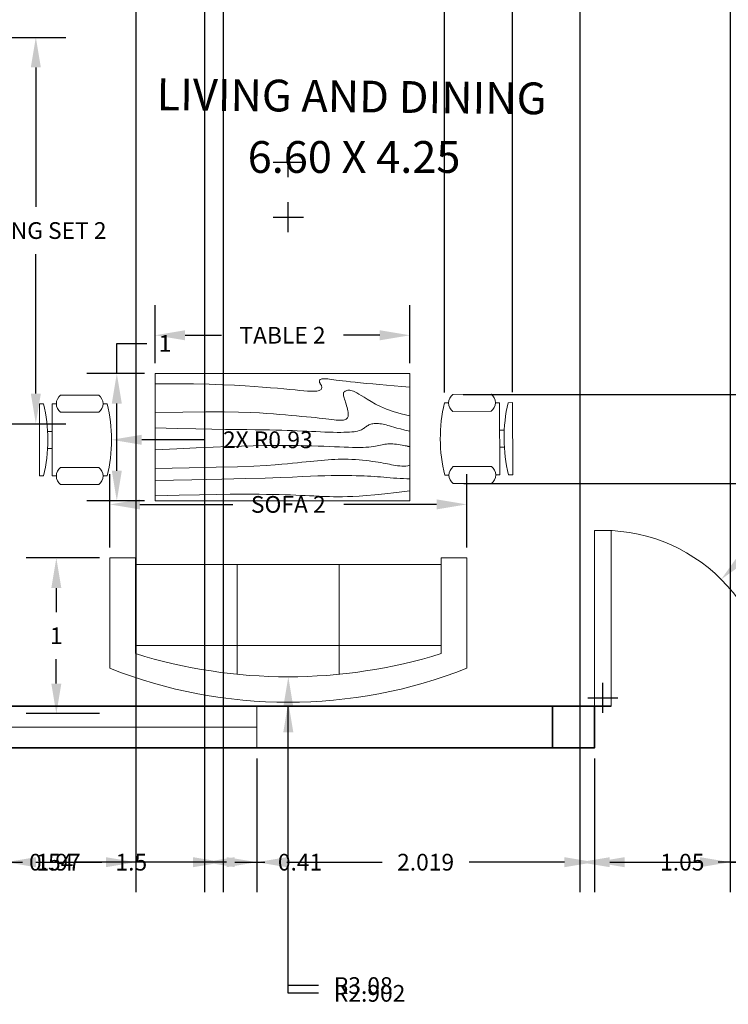
# Model space of a CAD drawing. Units: metres. Extents: x 180.3 to 196.1, y 135.7 to 166.1.
# Tile 2 of 5: x 183.3 to 187.5, y 150.2 to 156.1. Entities that reach past the tile are written whole.
import ezdxf

# ---------------------------------------------------------------- set-up
doc = ezdxf.new("R2010")
doc.units = ezdxf.units.M
doc.header["$MEASUREMENT"] = 0
for name, color, linetype, lineweight in [('A-ANNO-DIMS', 2, 'Continuous', 18), ('A-AREA-IDEN', 210, 'Continuous', 18), ('A-FURN', 190, 'Continuous', 18), ('A-GLAZ', 130, 'Continuous', 18), ('dim', 70, 'Continuous', 15), ('door', 240, 'Continuous', 18), ('wall', 50, 'Continuous', 35)]:
    doc.layers.add(name, color=color, linetype=linetype, lineweight=lineweight)
doc.styles.get("Standard").update_dxf_attribs({"font": 'arial.ttf', "height": 0.1})
doc.dimstyles.get("Standard").update_dxf_attribs({"dimtxt": 0.18, "dimasz": 0.18, "dimexe": 0.18, "dimexo": 0.0625, "dimgap": 0.09, "dimtad": 0, "dimtih": 1, "dimtoh": 1, "dimdec": 4, "dimzin": 0, "dimdsep": 46, "dimtxsty": 'Standard', "dimcen": 0.09, "dimadec": 0, "dimazin": 0, "dimtfac": 1, "dimtdec": 4, "dimtofl": 0, "dimtmove": 0, "dimatfit": 3, "dimfxl": 1, "dimtolj": 1, "dimtzin": 0, "dimarcsym": 0})

# ---------------------------------------------------------------- blocks, each defined once
blk = doc.blocks.new('Sofa - Roundback 7 ft.')
for p, q in [((-12.00002, -32.4421), (-12.00003, -6.5971)), ((11.99997, -32.4421), (11.99998, -6.5971)), ((-36.000027, -34), (-36.000027, -11.4696)), ((35.99998, -34), (35.99998, -11.4696)), ((-35.999844, -13.3819), (35.9998, -13.3819)), ((-36.000027, -32.4421), (35.99998, -32.4421))]:
    blk.add_line(p, q)
for points in [[(-36.000027, -34), (-42.000027, -34), (-42.000027, -8)], [(41.99998, -8), (41.99998, -34), (35.99998, -34)]]:
    blk.add_lwpolyline(points)
for centre, radius, start, end in [((0, -114.25), 114.25, 68.43141, 111.5686), ((-0.00001, -127.1968), 121.1968, 72.72033, 107.2797)]:
    blk.add_arc(centre, radius, start, end)
blk = doc.blocks.new('Table - Rectangular Woodgrain 60 x 30 in.')
for p, q in [((0, 0), (0, -30)), ((60, 0), (0, 0)), ((60, -30), (60, 0)), ((0, -30), (60, -30))]:
    blk.add_line(p, q)
for points in [[(0, -2.4), (4.8155, -2.418), (9.0302, -2.4688), (12.709, -2.5477), (15.9167, -2.65), (18.7181, -2.7711), (21.1781, -2.9063), (23.3616, -3.0508), (25.3333, -3.2), (27.1477, -3.3495), (28.8172, -3.4958), (30.3437, -3.636), (31.7291, -3.7667), (32.9756, -3.8849), (34.0849, -3.9875), (35.059, -4.0714), (35.9, -4.1334), (36.6114, -4.1711), (37.2041, -4.1854), (37.6906, -4.1779), (38.0833, -4.15), (38.3948, -4.1034), (38.6375, -4.0396), (38.8239, -3.9602), (38.9666, -3.8667), (39.0764, -3.7608), (39.1573, -3.6448), (39.2116, -3.521), (39.2416, -3.3917), (39.2498, -3.2593), (39.2385, -3.1261), (39.21, -2.9944), (39.1666, -2.8667), (39.111, -2.7447), (39.0468, -2.6281), (38.978, -2.5163), (38.9083, -2.4083), (38.8418, -2.3035), (38.7823, -2.201), (38.7337, -2.1001), (38.7, -2), (38.6844, -1.9003), (38.6875, -1.8021), (38.7094, -1.707), (38.75, -1.6167), (38.8094, -1.5326), (38.8875, -1.4563), (38.9844, -1.3893), (39.1, -1.3333), (39.2351, -1.2896), (39.3937, -1.2583), (39.5804, -1.2396), (39.8, -1.2333), (40.057, -1.2396), (40.3562, -1.2583), (40.7023, -1.2896), (41.1, -1.3333), (41.5547, -1.3895), (42.0755, -1.4573), (42.6721, -1.5361), (43.3542, -1.625), (44.1316, -1.7233), (45.014, -1.8302), (46.0114, -1.9449), (47.1333, -2.0667), (48.3862, -2.1947), (49.7625, -2.3281), (51.2513, -2.4663), (52.8416, -2.6083), (54.5226, -2.7535), (56.2833, -2.9011), (58.1127, -3.0501), (60, -3.2)], [(0, -9.2), (6.5759, -9.0858), (11.9385, -9.0365), (16.2527, -9.0418), (19.6833, -9.0917), (22.3952, -9.1759), (24.5531, -9.2844), (26.322, -9.4069), (27.8666, -9.5333), (29.3241, -9.6553), (30.7203, -9.7719), (32.0532, -9.8837), (33.3208, -9.9917), (34.5213, -10.0965), (35.6526, -10.199), (36.7128, -10.2999), (37.7, -10.4), (38.6129, -10.4996), (39.4531, -10.5969), (40.223, -10.6895), (40.925, -10.775), (41.5613, -10.8512), (42.1344, -10.9156), (42.6465, -10.966), (43.1, -11), (43.4976, -11.0158), (43.8437, -11.0136), (44.143, -10.9942), (44.4, -10.9583), (44.6195, -10.9069), (44.8062, -10.8406), (44.9648, -10.7603), (45.1, -10.6667), (45.2155, -10.5598), (45.3114, -10.4365), (45.3871, -10.2929), (45.4416, -10.125), (45.4743, -9.929), (45.4844, -9.7011), (45.4709, -9.4371), (45.4333, -9.1333), (45.3716, -8.7883), (45.2896, -8.4104), (45.1919, -8.0107), (45.0833, -7.6), (44.9685, -7.1893), (44.8521, -6.7896), (44.7388, -6.4117), (44.6333, -6.0667), (44.54, -5.7628), (44.4614, -5.4979), (44.4001, -5.2675), (44.3583, -5.0667), (44.3384, -4.8909), (44.3427, -4.7354), (44.3736, -4.5956), (44.4333, -4.4667), (44.5236, -4.3453), (44.6427, -4.2333), (44.7884, -4.1339), (44.9583, -4.05), (45.1501, -3.9849), (45.3614, -3.9417), (45.59, -3.9234), (45.8333, -3.9333), (46.0915, -3.9749), (46.3734, -4.0531), (46.6906, -4.1736), (47.0542, -4.3417), (47.4756, -4.5629), (47.9661, -4.8427), (48.5372, -5.1866), (49.2, -5.6), (49.9676, -6.0844), (50.8594, -6.625), (51.8965, -7.2031), (53.1, -7.8), (54.491, -8.3969), (56.0906, -8.975), (57.9199, -9.5156), (60, -10)], [(0, -12.8), (5.1847, -12.9322), (9.6213, -13.0323), (13.3963, -13.1059), (16.5958, -13.1583), (19.3063, -13.1952), (21.614, -13.2219), (23.6054, -13.2439), (25.3666, -13.2667), (26.9728, -13.2947), (28.4531, -13.3281), (29.8256, -13.3663), (31.1083, -13.4083), (32.3191, -13.4535), (33.476, -13.501), (34.597, -13.5501), (35.7, -13.6), (36.7984, -13.6497), (37.8875, -13.6979), (38.9578, -13.743), (40, -13.7833), (41.0047, -13.8174), (41.9625, -13.8438), (42.864, -13.8607), (43.7, -13.8667), (44.4631, -13.8604), (45.1552, -13.8417), (45.7801, -13.8104), (46.3416, -13.7667), (46.8439, -13.7104), (47.2906, -13.6417), (47.6858, -13.5604), (48.0333, -13.4667), (48.3375, -13.3608), (48.6042, -13.2448), (48.8396, -13.121), (49.05, -12.9917), (49.2417, -12.8593), (49.4208, -12.7261), (49.5937, -12.5944), (49.7667, -12.4667), (49.9452, -12.3451), (50.1323, -12.2313), (50.3303, -12.1268), (50.5416, -12.0333), (50.7686, -11.9524), (51.0135, -11.8854), (51.2788, -11.8341), (51.5666, -11.8), (51.8785, -11.7843), (52.2116, -11.7865), (52.562, -11.8059), (52.926, -11.8417), (53.2998, -11.8931), (53.6795, -11.9594), (54.0614, -12.0397), (54.4416, -12.1333), (54.8223, -12.2401), (55.2293, -12.3625), (55.6942, -12.5037), (56.2489, -12.6667), (56.9251, -12.8547), (57.7545, -13.0708), (58.7689, -13.3182), (60, -13.6)], [(0, -18), (5.124, -17.7273), (9.6609, -17.5057), (13.6705, -17.3303), (17.2125, -17.1958), (20.3467, -17.0973), (23.1328, -17.0297), (25.6307, -16.9878), (27.9, -16.9667), (29.9928, -16.9617), (31.9302, -16.9703), (33.7254, -16.9907), (35.3917, -17.0208), (36.9423, -17.0588), (38.3906, -17.1026), (39.7499, -17.1503), (41.0333, -17.2), (42.2519, -17.2496), (43.4073, -17.2969), (44.4986, -17.3395), (45.525, -17.375), (46.4858, -17.4012), (47.3802, -17.4156), (48.2074, -17.416), (48.9667, -17.4), (49.6583, -17.3662), (50.2872, -17.3167), (50.8595, -17.2547), (51.3812, -17.1833), (51.8584, -17.1057), (52.2971, -17.025), (52.7034, -16.9443), (53.0833, -16.8667), (53.443, -16.7951), (53.789, -16.7313), (54.128, -16.6768), (54.4666, -16.6334), (54.8115, -16.6024), (55.1693, -16.5854), (55.5465, -16.5841), (55.95, -16.6), (56.3828, -16.6337), (56.8346, -16.6823), (57.2915, -16.7418), (57.7396, -16.8084), (58.165, -16.878), (58.5539, -16.9469), (58.8924, -17.0111), (59.1666, -17.0667), (59.3679, -17.1107), (59.5078, -17.1438), (59.6032, -17.1675), (59.6708, -17.1833), (59.7275, -17.193), (59.7901, -17.1979), (59.8753, -17.1998), (60, -17.2)], [(0, -22.4), (8.0098, -22.2501), (14.4094, -22.1011), (19.4168, -21.9535), (23.25, -21.8083), (26.1269, -21.6663), (28.2656, -21.5281), (29.884, -21.3947), (31.2, -21.2667), (32.3967, -21.1448), (33.5172, -21.0292), (34.5697, -20.9198), (35.5625, -20.8167), (36.5037, -20.7198), (37.4015, -20.6292), (38.2642, -20.5448), (39.1, -20.4667), (39.9164, -20.3951), (40.7187, -20.3313), (41.5117, -20.2768), (42.3, -20.2333), (43.0883, -20.2024), (43.8812, -20.1854), (44.6836, -20.1841), (45.5, -20.2), (46.3328, -20.234), (47.1747, -20.2844), (48.0163, -20.3488), (48.8479, -20.425), (49.66, -20.5106), (50.4429, -20.6031), (51.1872, -20.7004), (51.8833, -20.8), (52.5246, -20.8999), (53.1166, -20.9995), (53.6681, -21.0983), (54.1875, -21.1958), (54.6834, -21.2919), (55.1646, -21.3859), (55.6394, -21.4777), (56.1167, -21.5667), (56.6028, -21.6515), (57.0961, -21.7266), (57.5929, -21.7852), (58.0896, -21.8208), (58.5823, -21.8268), (59.0674, -21.7964), (59.5412, -21.723), (60, -21.6)], [(0, -25.2), (8.6355, -25.0504), (15.7026, -24.9031), (21.4049, -24.7606), (25.9458, -24.625), (29.529, -24.4988), (32.3578, -24.3844), (34.6359, -24.284), (36.5667, -24.2), (38.3213, -24.1341), (39.9417, -24.0854), (41.437, -24.0523), (42.8167, -24.0333), (44.0901, -24.0268), (45.2667, -24.0313), (46.3557, -24.0451), (47.3667, -24.0667), (48.309, -24.0947), (49.1928, -24.1287), (50.0284, -24.168), (50.826, -24.2125), (51.5959, -24.2617), (52.3483, -24.3151), (53.0935, -24.3725), (53.8417, -24.4334), (54.6009, -24.497), (55.3699, -24.561), (56.1454, -24.6226), (56.9239, -24.6792), (57.7021, -24.7279), (58.4764, -24.7662), (59.2435, -24.7911), (60, -24.8)], [(0, -28.8), (5.6867, -28.6681), (10.45, -28.5698), (14.407, -28.5012), (17.675, -28.4584), (20.3711, -28.4374), (22.6125, -28.4344), (24.5164, -28.4455), (26.2, -28.4667), (27.762, -28.4947), (29.2276, -28.5281), (30.6033, -28.5663), (31.8958, -28.6084), (33.1118, -28.6535), (34.2578, -28.7011), (35.3405, -28.7501), (36.3666, -28.8), (37.3443, -28.8497), (38.288, -28.8974), (39.2137, -28.9412), (40.1375, -28.9792), (41.0753, -29.0093), (42.0432, -29.0297), (43.0572, -29.0384), (44.1333, -29.0333), (45.2936, -29.0114), (46.5843, -28.9641), (48.0579, -28.8816), (49.7666, -28.7542), (51.7629, -28.5721), (54.0989, -28.3255), (56.8272, -28.0048), (60, -27.6)]]:
    blk.add_lwpolyline(points)
blk = doc.blocks.new('Chair - Desk')
for p, q in [((-8.5, 0), (-8.5, -1)), ((-8.5, 0), (8.5, 0)), ((8.5, 0), (8.5, -1)), ((-2, -3), (-2, -1.9355)), ((2, -1.9576), (2, -3)), ((-8.5, -3), (-8.5, -4)), ((-8.5, -3), (8.5, -3)), ((8.5, -3), (8.5, -4)), ((-10.5, -5), (-10.5, -14)), ((-6.5, -14), (-6.5, -5)), ((6.5, -5), (6.5, -14)), ((10.5, -14), (10.5, -5)), ((-8.5, -15), (-8.5, -16)), ((8.5, -15), (8.5, -16))]:
    blk.add_line(p, q)
for centre, radius, start, end in [((0, 34.625), 36.625, 256.5803, 283.4197), ((-8.5, -6.5), 2.5, 36.8699, 143.1301), ((8.5, -6.5), 2.5, 36.8699, 143.1301), ((-8.5, -12.5), 2.5, 216.8699, 323.1301), ((0, 19.625), 36.625, 256.5803, 283.4197), ((8.5, -12.5), 2.5, 216.8699, 323.1301)]:
    blk.add_arc(centre, radius, start, end)
blk = doc.blocks.new('DOOR-1050')
for p, q in [((0.0004, -0.0001), (0.0004, 1.0499)), ((0.1004, -0.0001), (0.1004, 1.0499))]:
    blk.add_line(p, q)
blk.add_arc((0.0504, 0.0499), 1.0012, 357.13759, 92.86241)
blk = doc.blocks.new('WIN-1500')
for p, q in [((0.0003, 0.2499), (0.0003, -0.0001)), ((1.5003, 0.2499), (1.5003, -0.0001)), ((1.5003, 0.1249), (0.0003, 0.1249))]:
    blk.add_line(p, q)
blk = doc.blocks.new('*D25')
at = {"layer": 'A-ANNO-DIMS', "color": 0, "lineweight": -2, "transparency": 16777216}
for p, q in [((183.1113, 155.9984), (183.5755, 155.9984)), ((183.3955, 155.8184), (183.3955, 154.9844)), ((183.3955, 153.867), (183.3955, 154.701)), ((183.1113, 153.687), (183.5755, 153.687))]:
    blk.add_line(p, q, dxfattribs=at)
at = {"layer": 'A-ANNO-DIMS', "color": 0, "transparency": 16777216}
for points in [[(183.3655, 155.8184), (183.4255, 155.8184), (183.3955, 155.9984)], [(183.3655, 153.867), (183.4255, 153.867), (183.3955, 153.687)]]:
    blk.add_solid(points, dxfattribs=at)
at = {"layer": 'Defpoints', "color": 0, "transparency": 16777216}
for p in [(183.0488, 155.9984), (183.0488, 153.687), (183.3955, 153.687)]:
    blk.add_point(p, dxfattribs=at)
at = {"layer": 'A-ANNO-DIMS', "color": 0, "transparency": 16777216, "insert": (183.3955, 154.8427), "char_height": 0.1, "attachment_point": 5}
blk.add_mtext('\\A1;DINING SET 2', dxfattribs=at)
blk = doc.blocks.new('*D27')
at = {"layer": 'A-ANNO-DIMS', "color": 0, "lineweight": -2, "transparency": 16777216}
for p, q in [((183.8381, 152.9469), (183.8381, 153.3845)), ((185.9717, 152.9469), (185.9717, 153.3845)), ((184.0181, 153.2045), (184.5733, 153.2045)), ((185.7917, 153.2045), (185.2365, 153.2045))]:
    blk.add_line(p, q, dxfattribs=at)
at = {"layer": 'A-ANNO-DIMS', "color": 0, "transparency": 16777216}
for points in [[(184.0181, 153.2345), (184.0181, 153.1745), (183.8381, 153.2045)], [(185.7917, 153.2345), (185.7917, 153.1745), (185.9717, 153.2045)]]:
    blk.add_solid(points, dxfattribs=at)
at = {"layer": 'Defpoints', "color": 0, "transparency": 16777216}
for p in [(183.8381, 153.2045), (183.8381, 152.8844), (185.9717, 152.8844)]:
    blk.add_point(p, dxfattribs=at)
at = {"layer": 'A-ANNO-DIMS', "color": 0, "transparency": 16777216, "insert": (184.9049, 153.2045), "char_height": 0.1, "attachment_point": 5}
blk.add_mtext('\\A1;SOFA 2', dxfattribs=at)
blk = doc.blocks.new('*D28')
at = {"layer": 'A-ANNO-DIMS', "color": 0, "lineweight": -2, "transparency": 16777216}
for p, q in [((183.7756, 152.8844), (183.3381, 152.8844)), ((183.5181, 152.7044), (183.5181, 152.559)), ((183.5181, 152.1331), (183.5181, 152.2786)), ((183.7756, 151.9531), (183.3381, 151.9531))]:
    blk.add_line(p, q, dxfattribs=at)
at = {"layer": 'A-ANNO-DIMS', "color": 0, "transparency": 16777216}
for points in [[(183.4881, 152.7044), (183.5481, 152.7044), (183.5181, 152.8844)], [(183.4881, 152.1331), (183.5481, 152.1331), (183.5181, 151.9531)]]:
    blk.add_solid(points, dxfattribs=at)
at = {"layer": 'Defpoints', "color": 0, "transparency": 16777216}
for p in [(183.8381, 152.8844), (183.5181, 151.9531), (183.8381, 151.9531)]:
    blk.add_point(p, dxfattribs=at)
at = {"layer": 'A-ANNO-DIMS', "color": 0, "transparency": 16777216, "insert": (183.5181, 152.4188), "char_height": 0.1, "attachment_point": 5}
blk.add_mtext('\\A1;1', dxfattribs=at)
blk = doc.blocks.new('*D29')
at = {"layer": 'A-ANNO-DIMS', "color": 0, "lineweight": -2, "transparency": 16777216}
for p, q in [((184.1082, 154.0502), (184.1082, 154.3963)), ((185.6322, 154.0502), (185.6322, 154.3963)), ((184.2882, 154.2163), (184.506, 154.2163)), ((185.4522, 154.2163), (185.2345, 154.2163))]:
    blk.add_line(p, q, dxfattribs=at)
at = {"layer": 'A-ANNO-DIMS', "color": 0, "transparency": 16777216}
for points in [[(184.2882, 154.2463), (184.2882, 154.1863), (184.1082, 154.2163)], [(185.4522, 154.2463), (185.4522, 154.1863), (185.6322, 154.2163)]]:
    blk.add_solid(points, dxfattribs=at)
at = {"layer": 'Defpoints', "color": 0, "transparency": 16777216}
for p in [(185.6322, 154.2163), (184.1082, 153.9877), (185.6322, 153.9877)]:
    blk.add_point(p, dxfattribs=at)
at = {"layer": 'A-ANNO-DIMS', "color": 0, "transparency": 16777216, "insert": (184.8702, 154.2163), "char_height": 0.1, "attachment_point": 5}
blk.add_mtext('\\A1;TABLE 2', dxfattribs=at)
blk = doc.blocks.new('*D30')
at = {"layer": 'A-ANNO-DIMS', "color": 0, "lineweight": -2, "transparency": 16777216}
for p, q in [((183.8796, 153.9877), (183.8796, 154.1677)), ((183.8796, 154.1677), (184.0596, 154.1677)), ((184.0457, 153.9877), (183.6996, 153.9877)), ((183.8796, 153.4057), (183.8796, 153.8077)), ((184.0457, 153.2257), (183.6996, 153.2257))]:
    blk.add_line(p, q, dxfattribs=at)
at = {"layer": 'A-ANNO-DIMS', "color": 0, "transparency": 16777216}
for points in [[(183.8496, 153.8077), (183.9096, 153.8077), (183.8796, 153.9877)], [(183.8496, 153.4057), (183.9096, 153.4057), (183.8796, 153.2257)]]:
    blk.add_solid(points, dxfattribs=at)
at = {"layer": 'Defpoints', "color": 0, "transparency": 16777216}
for p in [(183.8796, 153.9877), (184.1082, 153.9877), (184.1082, 153.2257)]:
    blk.add_point(p, dxfattribs=at)
at = {"layer": 'A-ANNO-DIMS', "color": 0, "transparency": 16777216, "insert": (184.1681, 154.1677), "char_height": 0.1, "attachment_point": 5}
blk.add_mtext('\\A1;1', dxfattribs=at)
blk = doc.blocks.new('*D40')
at = {"layer": 'A-ANNO-DIMS', "color": 0, "lineweight": -2, "transparency": 16777216}
for p, q in [((183.2164, 151.6854), (183.2164, 150.8842)), ((184.7164, 151.6854), (184.7164, 150.8842)), ((183.3964, 151.0642), (183.7897, 151.0642)), ((184.5364, 151.0642), (184.1431, 151.0642))]:
    blk.add_line(p, q, dxfattribs=at)
at = {"layer": 'A-ANNO-DIMS', "color": 0, "transparency": 16777216}
for points in [[(183.3964, 151.0942), (183.3964, 151.0342), (183.2164, 151.0642)], [(184.5364, 151.0942), (184.5364, 151.0342), (184.7164, 151.0642)]]:
    blk.add_solid(points, dxfattribs=at)
at = {"layer": 'Defpoints', "color": 0, "transparency": 16777216}
for p in [(183.2164, 151.7479), (184.7164, 151.7479), (184.7164, 151.0642)]:
    blk.add_point(p, dxfattribs=at)
at = {"layer": 'A-ANNO-DIMS', "color": 0, "transparency": 16777216, "insert": (183.9664, 151.0642), "char_height": 0.1, "attachment_point": 5}
blk.add_mtext('\\A1;1.5', dxfattribs=at)
blk = doc.blocks.new('*D41')
at = {"layer": 'A-ANNO-DIMS', "color": 0, "lineweight": -2, "transparency": 16777216}
for p, q in [((184.7164, 151.6854), (184.7164, 150.8842)), ((186.7354, 151.6854), (186.7354, 150.8842)), ((184.8964, 151.0642), (185.4662, 151.0642)), ((186.5554, 151.0642), (185.9856, 151.0642))]:
    blk.add_line(p, q, dxfattribs=at)
at = {"layer": 'A-ANNO-DIMS', "color": 0, "transparency": 16777216}
for points in [[(184.8964, 151.0942), (184.8964, 151.0342), (184.7164, 151.0642)], [(186.5554, 151.0942), (186.5554, 151.0342), (186.7354, 151.0642)]]:
    blk.add_solid(points, dxfattribs=at)
at = {"layer": 'Defpoints', "color": 0, "transparency": 16777216}
for p in [(184.7164, 151.7479), (186.7354, 151.7479), (186.7354, 151.0642)]:
    blk.add_point(p, dxfattribs=at)
at = {"layer": 'A-ANNO-DIMS', "color": 0, "transparency": 16777216, "insert": (185.7259, 151.0642), "char_height": 0.1, "attachment_point": 5}
blk.add_mtext('\\A1;2.019', dxfattribs=at)
blk = doc.blocks.new('*D42')
at = {"layer": 'A-ANNO-DIMS', "color": 0, "lineweight": -2, "transparency": 16777216}
for p, q in [((186.7354, 151.6854), (186.7354, 150.8842)), ((187.7854, 151.6854), (187.7854, 150.8842)), ((186.9154, 151.0642), (187.0449, 151.0642)), ((187.6054, 151.0642), (187.476, 151.0642))]:
    blk.add_line(p, q, dxfattribs=at)
at = {"layer": 'A-ANNO-DIMS', "color": 0, "transparency": 16777216}
for points in [[(186.9154, 151.0942), (186.9154, 151.0342), (186.7354, 151.0642)], [(187.6054, 151.0942), (187.6054, 151.0342), (187.7854, 151.0642)]]:
    blk.add_solid(points, dxfattribs=at)
at = {"layer": 'Defpoints', "color": 0, "transparency": 16777216}
for p in [(186.7354, 151.7479), (187.7854, 151.7479), (187.7854, 151.0642)]:
    blk.add_point(p, dxfattribs=at)
at = {"layer": 'A-ANNO-DIMS', "color": 0, "transparency": 16777216, "insert": (187.2604, 151.0642), "char_height": 0.1, "attachment_point": 5}
blk.add_mtext('\\A1;1.05', dxfattribs=at)
blk = doc.blocks.new('*D51')
at = {"layer": 'A-ANNO-DIMS', "color": 0, "lineweight": -2, "transparency": 16777216}
for p, q in [((182.5473, 156.4354), (182.5473, 150.8842)), ((183.0878, 156.4354), (183.0878, 150.8842)), ((182.7273, 151.0642), (182.9078, 151.0642)), ((183.0878, 151.0642), (183.2678, 151.0642))]:
    blk.add_line(p, q, dxfattribs=at)
at = {"layer": 'A-ANNO-DIMS', "color": 0, "transparency": 16777216}
for points in [[(182.7273, 151.0942), (182.7273, 151.0342), (182.5473, 151.0642)], [(182.9078, 151.0942), (182.9078, 151.0342), (183.0878, 151.0642)]]:
    blk.add_solid(points, dxfattribs=at)
at = {"layer": 'Defpoints', "color": 0, "transparency": 16777216}
for p in [(182.5473, 156.4979), (183.0878, 156.4979), (183.0878, 151.0642)]:
    blk.add_point(p, dxfattribs=at)
at = {"layer": 'A-ANNO-DIMS', "color": 0, "transparency": 16777216, "insert": (183.4875, 151.0642), "char_height": 0.1, "attachment_point": 5}
blk.add_mtext('\\A1;0.54', dxfattribs=at)
blk = doc.blocks.new('*D52')
at = {"layer": 'A-ANNO-DIMS', "color": 0, "lineweight": -2, "transparency": 16777216}
for p, q in [((182.5473, 158.3772), (182.5473, 150.8842)), ((184.5151, 158.3772), (184.5151, 150.8842)), ((182.7273, 151.0642), (183.316, 151.0642)), ((184.3351, 151.0642), (183.7464, 151.0642))]:
    blk.add_line(p, q, dxfattribs=at)
at = {"layer": 'A-ANNO-DIMS', "color": 0, "transparency": 16777216}
for points in [[(182.7273, 151.0942), (182.7273, 151.0342), (182.5473, 151.0642)], [(184.3351, 151.0942), (184.3351, 151.0342), (184.5151, 151.0642)]]:
    blk.add_solid(points, dxfattribs=at)
at = {"layer": 'Defpoints', "color": 0, "transparency": 16777216}
for p in [(182.5473, 158.4397), (184.5151, 158.4397), (184.5151, 151.0642)]:
    blk.add_point(p, dxfattribs=at)
at = {"layer": 'A-ANNO-DIMS', "color": 0, "transparency": 16777216, "insert": (183.5312, 151.0642), "char_height": 0.1, "attachment_point": 5}
blk.add_mtext('\\A1;1.97', dxfattribs=at)
blk = doc.blocks.new('*D54')
at = {"layer": 'A-ANNO-DIMS', "color": 0, "lineweight": -2, "transparency": 16777216}
for p, q in [((186.6473, 162.1854), (186.6473, 150.8842)), ((187.5473, 162.1854), (187.5473, 150.8842)), ((186.8273, 151.0642), (187.3673, 151.0642)), ((187.5473, 151.0642), (187.7273, 151.0642))]:
    blk.add_line(p, q, dxfattribs=at)
at = {"layer": 'A-ANNO-DIMS', "color": 0, "transparency": 16777216}
for points in [[(186.8273, 151.0942), (186.8273, 151.0342), (186.6473, 151.0642)], [(187.3673, 151.0942), (187.3673, 151.0342), (187.5473, 151.0642)]]:
    blk.add_solid(points, dxfattribs=at)
at = {"layer": 'Defpoints', "color": 0, "transparency": 16777216}
for p in [(186.6473, 162.2479), (187.5473, 162.2479), (187.5473, 151.0642)]:
    blk.add_point(p, dxfattribs=at)
at = {"layer": 'A-ANNO-DIMS', "color": 0, "transparency": 16777216, "insert": (187.9085, 151.0642), "char_height": 0.1, "attachment_point": 5}
blk.add_mtext('\\A1;0.9', dxfattribs=at)
blk = doc.blocks.new('*D61')
at = {"layer": 'A-ANNO-DIMS', "color": 0, "lineweight": -2, "transparency": 16777216}
for p, q in [((183.9941, 158.6956), (183.9941, 150.8842)), ((184.4049, 158.6956), (184.4049, 150.8842)), ((183.8141, 151.0642), (183.6341, 151.0642)), ((184.5849, 151.0642), (184.7649, 151.0642))]:
    blk.add_line(p, q, dxfattribs=at)
at = {"layer": 'A-ANNO-DIMS', "color": 0, "transparency": 16777216}
for points in [[(183.8141, 151.0942), (183.8141, 151.0342), (183.9941, 151.0642)], [(184.5849, 151.0942), (184.5849, 151.0342), (184.4049, 151.0642)]]:
    blk.add_solid(points, dxfattribs=at)
at = {"layer": 'Defpoints', "color": 0, "transparency": 16777216}
for p in [(183.9941, 158.7581), (184.4049, 158.7581), (184.4049, 151.0642)]:
    blk.add_point(p, dxfattribs=at)
at = {"layer": 'A-ANNO-DIMS', "color": 0, "transparency": 16777216, "insert": (184.9751, 151.0642), "char_height": 0.1, "attachment_point": 5}
blk.add_mtext('\\A1;0.41', dxfattribs=at)
blk = doc.blocks.new('*D63')
at = {"layer": 'A-ANNO-DIMS', "color": 0, "lineweight": -2, "transparency": 16777216}
for p, q in [((185.8382, 153.8738), (185.8382, 166.1117)), ((186.2446, 153.8757), (186.2446, 166.1117)), ((185.6582, 165.9317), (185.4782, 165.9317)), ((186.4246, 165.9317), (186.6046, 165.9317))]:
    blk.add_line(p, q, dxfattribs=at)
at = {"layer": 'A-ANNO-DIMS', "color": 0, "transparency": 16777216}
for points in [[(185.6582, 165.9617), (185.6582, 165.9017), (185.8382, 165.9317)], [(186.4246, 165.9617), (186.4246, 165.9017), (186.2446, 165.9317)]]:
    blk.add_solid(points, dxfattribs=at)
at = {"layer": 'Defpoints', "color": 0, "transparency": 16777216}
for p in [(186.2446, 165.9317), (185.8382, 153.8113), (186.2446, 153.8132)]:
    blk.add_point(p, dxfattribs=at)
at = {"layer": 'A-ANNO-DIMS', "color": 0, "transparency": 16777216, "insert": (186.8148, 165.9317), "char_height": 0.1, "attachment_point": 5}
blk.add_mtext('\\A1;0.41', dxfattribs=at)
blk = doc.blocks.new('*D64')
at = {"layer": 'A-ANNO-DIMS', "color": 0, "lineweight": -2, "transparency": 16777216}
for p, q in [((195.531085, 154.042344), (195.531085, 154.222344)), ((185.951216, 153.862344), (195.711085, 153.862344)), ((185.953765, 153.32895), (195.711085, 153.32895)), ((195.531085, 153.14895), (195.531085, 152.96895))]:
    blk.add_line(p, q, dxfattribs=at)
at = {"layer": 'A-ANNO-DIMS', "color": 0, "transparency": 16777216}
for points in [[(195.501085, 154.042344), (195.561085, 154.042344), (195.531085, 153.862344)], [(195.501085, 153.14895), (195.561085, 153.14895), (195.531085, 153.32895)]]:
    blk.add_solid(points, dxfattribs=at)
at = {"layer": 'Defpoints', "color": 0, "transparency": 16777216}
for p in [(185.888716, 153.862344), (195.531085, 153.862344), (185.891265, 153.32895)]:
    blk.add_point(p, dxfattribs=at)
at = {"layer": 'A-ANNO-DIMS', "color": 0, "transparency": 16777216, "insert": (195.531085, 153.595647), "char_height": 0.1, "attachment_point": 5}
blk.add_mtext('\\A1;0.53', dxfattribs=at)
blk = doc.blocks.new('*D66')
at = {"layer": 'A-ANNO-DIMS', "color": 0, "lineweight": -2, "transparency": 16777216}
for p, q in [((187.9178, 153.1811), (187.6204, 152.8835)), ((188.0978, 153.1811), (187.9178, 153.1811)), ((186.7854, 151.9579), (186.7854, 152.1379)), ((186.6954, 152.0479), (186.8754, 152.0479))]:
    blk.add_line(p, q, dxfattribs=at)
at = {"layer": 'A-ANNO-DIMS', "color": 0, "transparency": 16777216}
blk.add_solid([(187.5992, 152.9047), (187.6416, 152.8623), (187.4932, 152.7562)], dxfattribs=at)
at = {"layer": 'Defpoints', "color": 0, "transparency": 16777216}
for p in [(187.4932, 152.7562), (186.7854, 152.0479)]:
    blk.add_point(p, dxfattribs=at)
at = {"layer": 'A-ANNO-DIMS', "color": 0, "transparency": 16777216, "insert": (188.4748, 153.1811), "char_height": 0.1, "attachment_point": 5}
blk.add_mtext('\\A1;4X R1.00', dxfattribs=at)
blk = doc.blocks.new('*D69')
at = {"layer": 'A-ANNO-DIMS', "color": 0, "lineweight": -2, "transparency": 16777216}
for p, q in [((182.9181, 153.5006), (182.9181, 153.6806)), ((182.8281, 153.5906), (183.0081, 153.5906)), ((184.4065, 153.5912), (184.0284, 153.5911))]:
    blk.add_line(p, q, dxfattribs=at)
at = {"layer": 'A-ANNO-DIMS', "color": 0, "transparency": 16777216}
blk.add_solid([(184.0284, 153.6211), (184.0284, 153.5611), (183.8484, 153.591)], dxfattribs=at)
at = {"layer": 'Defpoints', "color": 0, "transparency": 16777216}
for p in [(182.9181, 153.5906), (183.8484, 153.591)]:
    blk.add_point(p, dxfattribs=at)
at = {"layer": 'A-ANNO-DIMS', "color": 0, "transparency": 16777216, "insert": (184.7826, 153.5912), "char_height": 0.1, "attachment_point": 5}
blk.add_mtext('\\A1;2X R0.93', dxfattribs=at)
blk = doc.blocks.new('*D70')
at = {"layer": 'A-ANNO-DIMS', "color": 0, "lineweight": -2, "transparency": 16777216}
for p, q in [((184.9049, 155.1616), (184.9049, 155.3416)), ((184.8149, 155.2516), (184.9949, 155.2516)), ((184.905, 150.3262), (184.905, 151.9932)), ((185.085, 150.3262), (184.905, 150.3262))]:
    blk.add_line(p, q, dxfattribs=at)
at = {"layer": 'A-ANNO-DIMS', "color": 0, "transparency": 16777216}
blk.add_solid([(184.935, 151.9932), (184.875, 151.9932), (184.905, 152.1732)], dxfattribs=at)
at = {"layer": 'Defpoints', "color": 0, "transparency": 16777216}
for p in [(184.9049, 155.2516), (184.905, 152.1732)]:
    blk.add_point(p, dxfattribs=at)
at = {"layer": 'A-ANNO-DIMS', "color": 0, "transparency": 16777216, "insert": (185.3529, 150.3262), "char_height": 0.1, "attachment_point": 5}
blk.add_mtext('\\A1;R3.08', dxfattribs=at)
blk = doc.blocks.new('*D71')
at = {"layer": 'A-ANNO-DIMS', "color": 0, "lineweight": -2, "transparency": 16777216}
for p, q in [((184.9049, 154.8328), (184.9049, 155.0128)), ((184.8149, 154.9228), (184.9949, 154.9228)), ((184.905, 150.2797), (184.905, 151.8408)), ((185.085, 150.2797), (184.905, 150.2797))]:
    blk.add_line(p, q, dxfattribs=at)
at = {"layer": 'A-ANNO-DIMS', "color": 0, "transparency": 16777216}
blk.add_solid([(184.935, 151.8408), (184.875, 151.8408), (184.905, 152.0208)], dxfattribs=at)
at = {"layer": 'Defpoints', "color": 0, "transparency": 16777216}
for p in [(184.9049, 154.9228), (184.905, 152.0208)]:
    blk.add_point(p, dxfattribs=at)
at = {"layer": 'A-ANNO-DIMS', "color": 0, "transparency": 16777216, "insert": (185.3911, 150.2797), "char_height": 0.1, "attachment_point": 5}
blk.add_mtext('\\A1;R2.902', dxfattribs=at)

msp = doc.modelspace()

# ---------------------------------------------------------------- linework, layer by layer
at = {"layer": 'wall'}
for p, q in [((186.8354, 151.9979), (181.4473, 151.9979)), ((186.7354, 151.7479), (181.1973, 151.7479))]:
    msp.add_line(p, q, dxfattribs=at)
msp.add_lwpolyline([(186.4854, 151.9979), (186.7354, 151.9979), (186.7354, 151.7479), (186.4854, 151.7479)], close=True, dxfattribs=at)

# ---------------------------------------------------------------- block references
at = {"layer": 'A-FURN', "xscale": 0.0254, "yscale": 0.0254, "zscale": 0.0254}
msp.add_blockref('Table - Rectangular Woodgrain 60 x 30 in.', (184.1082, 153.9877), dxfattribs=at)
at = {"layer": 'A-FURN', "yscale": 0.0254, "zscale": 0.0254}
for name, p, xscale, rotation in [('Chair - Desk', (183.4166, 153.5906), 0.0254, 90), ('Chair - Desk', (186.2456, 153.5973), -0.0254, 270.2737751839787), ('Sofa - Roundback 7 ft.', (184.9049, 152.0208), 0.0254, 180)]:
    msp.add_blockref(name, p, dxfattribs=dict(at, xscale=xscale, rotation=rotation))
at = {"layer": 'A-GLAZ'}
msp.add_blockref('WIN-1500', (183.216, 151.748), dxfattribs=at)
at = {"layer": 'door'}
msp.add_blockref('DOOR-1050', (186.735, 151.998), dxfattribs=at)

# ---------------------------------------------------------------- texts
at = {"layer": 'A-AREA-IDEN', "insert": (183.198, 155.7632), "char_height": 0.19, "attachment_point": 1, "rotation": 359.37384}
msp.add_mtext_dynamic_manual_height_columns('\\pxqc;LIVING AND DINING ', width=4.172977, gutter_width=1, heights=[0], dxfattribs=at)
at = {"layer": 'dim', "insert": (183.8767, 155.3779), "char_height": 0.19, "attachment_point": 1}
msp.add_mtext_dynamic_manual_height_columns('\\pxqc;6.60 X 4.25', width=2.842675, gutter_width=1, heights=[0], dxfattribs=at)

# ---------------------------------------------------------------- dimensions: what is measured, and where the dimension line sits
at = {"layer": 'A-ANNO-DIMS'}
for base, p1, p2, override, picture, middle in [((186.2446, 165.9317), (185.8382, 153.8113), (186.2446, 153.8132), {"dimdec": 2, "dimlfac": 1, "dimrnd": 0, "dimzin": 0, "dimdsep": 46, "dimlunit": 2}, '*D63', (186.8148, 165.9317)), ((187.5473, 151.0642), (186.6473, 162.2479), (187.5473, 162.2479), {"dimdec": 1, "dimlfac": 1, "dimrnd": 0, "dimzin": 0, "dimdsep": 46, "dimlunit": 2}, '*D54', (187.9085, 151.0642)), ((184.4049, 151.0642), (183.9941, 158.7581), (184.4049, 158.7581), {"dimdec": 2, "dimlfac": 1, "dimrnd": 0, "dimzin": 0, "dimdsep": 46, "dimlunit": 2}, '*D61', (184.9751, 151.0642)), ((184.5151, 151.0642), (182.5473, 158.4397), (184.5151, 158.4397), {"dimdec": 2, "dimlfac": 1, "dimrnd": 0, "dimzin": 0, "dimdsep": 46, "dimlunit": 2}, '*D52', (183.5312, 151.0642)), ((183.0878, 151.0642), (182.5473, 156.4979), (183.0878, 156.4979), {"dimdec": 2, "dimlfac": 1, "dimrnd": 0, "dimzin": 0, "dimdsep": 46, "dimlunit": 2}, '*D51', (183.4875, 151.0642)), ((184.7164, 151.0642), (183.2164, 151.7479), (184.7164, 151.7479), {"dimdec": 1, "dimlfac": 1, "dimrnd": 0, "dimzin": 0, "dimdsep": 46, "dimlunit": 2}, '*D40', (183.9664, 151.0642)), ((186.7354, 151.0642), (184.7164, 151.7479), (186.7354, 151.7479), {"dimdec": 3, "dimlfac": 1, "dimrnd": 0, "dimzin": 0, "dimdsep": 46, "dimlunit": 2}, '*D41', (185.7259, 151.0642)), ((187.7854, 151.0642), (186.7354, 151.7479), (187.7854, 151.7479), {"dimdec": 2, "dimlfac": 1, "dimrnd": 0, "dimzin": 0, "dimdsep": 46, "dimlunit": 2}, '*D42', (187.2604, 151.0642))]:
    dim = msp.add_linear_dim(base=base, p1=p1, p2=p2, dimstyle='Standard', override=override, dxfattribs=at)
    dim.commit()
    dim.dimension.update_dxf_attribs({"geometry": picture, "text_midpoint": middle})
for base, p1, p2, angle, text, picture, middle in [((183.3955, 153.687), (183.0488, 155.9984), (183.0488, 153.687), 270, 'DINING SET <>', '*D25', (183.3955, 154.8427)), ((183.8381, 153.2045), (185.9717, 152.8844), (183.8381, 152.8844), 180, 'SOFA <>', '*D27', (184.9049, 153.2045))]:
    dim = msp.add_linear_dim(base=base, p1=p1, p2=p2, angle=angle, text=text, dimstyle='Standard', override={"dimdec": 0, "dimlfac": 1, "dimrnd": 0, "dimzin": 0, "dimdsep": 46, "dimlunit": 2}, dxfattribs=at)
    dim.commit()
    dim.dimension.update_dxf_attribs({"geometry": picture, "text_midpoint": middle})
for center, mpoint, override, picture, middle in [((184.9049, 155.2516), (184.905, 152.1732), {"dimdec": 2, "dimlfac": 1, "dimrnd": 0, "dimzin": 0, "dimdsep": 46, "dimlunit": 2}, '*D70', (185.3529, 150.3262)), ((184.9049, 154.9228), (184.905, 152.0208), {"dimdec": 3, "dimlfac": 1, "dimrnd": 0, "dimzin": 0, "dimdsep": 46, "dimlunit": 2}, '*D71', (185.3911, 150.2797))]:
    dim = msp.add_radius_dim(center=center, mpoint=mpoint, dimstyle='Standard', override=override, dxfattribs=at)
    dim.commit()
    dim.dimension.update_dxf_attribs({"geometry": picture, "text_midpoint": middle, "dimtype": 164})
dim = msp.add_linear_dim(base=(185.6322, 154.2163), p1=(184.1082, 153.9877), p2=(185.6322, 153.9877), text='TABLE <>', dimstyle='Standard', override={"dimdec": 0, "dimlfac": 1, "dimrnd": 0, "dimzin": 0, "dimdsep": 46, "dimlunit": 2}, dxfattribs=at)
dim.commit()
dim.dimension.update_dxf_attribs({"geometry": '*D29', "text_midpoint": (184.8702, 154.2163)})
for base, p1, p2, angle, override, picture, middle in [((183.8796, 153.9877), (184.1082, 153.2257), (184.1082, 153.9877), 90, {"dimdec": 0, "dimlfac": 1, "dimrnd": 0, "dimzin": 0, "dimdsep": 46, "dimlunit": 2}, '*D30', (184.1681, 154.1677)), ((195.5311, 153.8623), (185.8913, 153.3289), (185.8887, 153.8623), 90, {"dimdec": 2, "dimlfac": 1, "dimrnd": 0, "dimzin": 0, "dimdsep": 46, "dimlunit": 2}, '*D64', (195.5311, 153.5956)), ((183.5181, 151.9531), (183.8381, 152.8844), (183.8381, 151.9531), 270, {"dimdec": 0, "dimlfac": 1, "dimrnd": 0, "dimzin": 0, "dimdsep": 46, "dimlunit": 2}, '*D28', (183.5181, 152.4188))]:
    dim = msp.add_linear_dim(base=base, p1=p1, p2=p2, angle=angle, dimstyle='Standard', override=override, dxfattribs=at)
    dim.commit()
    dim.dimension.update_dxf_attribs({"geometry": picture, "text_midpoint": middle})
for center, mpoint, text, picture, middle in [((182.9181, 153.5906), (183.8484, 153.591), '2X <>', '*D69', (184.4065, 153.5912)), ((186.7854, 152.0479), (187.4932, 152.7562), '4X <>', '*D66', (188.4748, 153.1811))]:
    dim = msp.add_radius_dim(center=center, mpoint=mpoint, text=text, dimstyle='Standard', override={"dimdec": 2, "dimlfac": 1, "dimrnd": 0, "dimzin": 0, "dimdsep": 46, "dimlunit": 2}, dxfattribs=at)
    dim.commit()
    dim.dimension.update_dxf_attribs({"geometry": picture, "text_midpoint": middle, "dimtype": 164})

doc.saveas('drawing.dxf')
